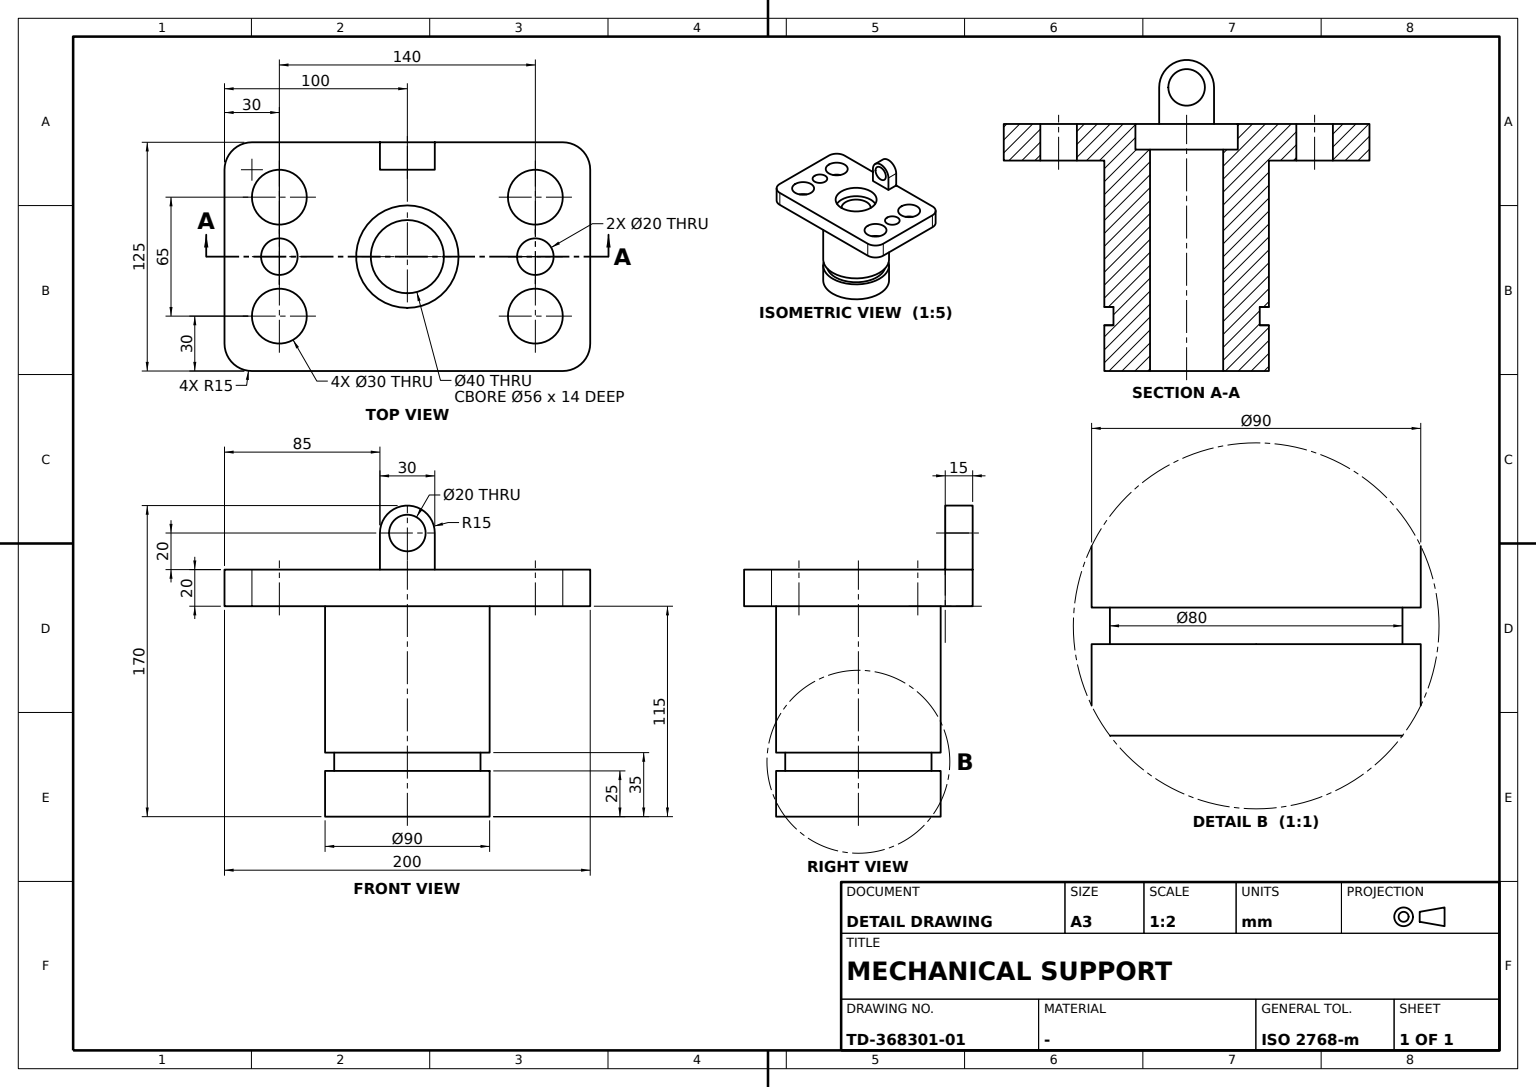
CATIA V5 part; units mm, degrees
sketch "Sketch1" plane through (0, 0, 0) normal (1, 0, 0) x (0, 1, 0)
  point P0 (20, 0)
  line L0 (20, 0) -> (20, 121)
  point P1 (45, 135)
  line L1 (45, 135) -> (45, 35)
  line L2 (45, 35) -> (40, 35)
  line L3 (40, 35) -> (40, 25)
  line L4 (40, 25) -> (45, 25)
  point P2 (45, 25)
  line L5 (45, 25) -> (45, 0)
  point P3 (45, 0)
  line L6 (45, 0) -> (20, 0)
  line L7 (20, 121) -> (28, 121)
  line L8 (28, 121) -> (28, 135)
  line L9 (28, 135) -> (45, 135)
  point P4 (45, 135)
  dimension "length L6" = 25
  dimension "distance L0 y axis" = 20
  dimension "length L5" = 25
  dimension "length L0" = 121
  dimension "length L3" = 10
  dimension "length L4" = 5
  dimension "distance L8 y axis" = 28
  dimension "distance L9 x axis" = 135
  constraint coincidence P0 x-axis
  constraint coincidence P2 L1
  constraint coincidence P3 x-axis
  constraint coincidence P4 L1
  constraint coincidence P1 P4
  constraint vertical L0 y-axis
  constraint vertical L1 y-axis
  constraint vertical L3 y-axis
  constraint vertical L5 y-axis
  constraint vertical L8 y-axis
  constraint horizontal L2 x-axis
  constraint horizontal L4 x-axis
  constraint horizontal L6 x-axis
  constraint horizontal L7 x-axis
  constraint horizontal L9 x-axis
revolve "Shaft1" add sketch "Sketch1" angle 360 about axis through (0, 0, 0) along (0, 0, 1)
sketch "Sketch2" plane through (0, 0, 135) normal (0, 0, 1) x (1, 0, 0)
  line L0 (100, 47.5) -> (100, -47.5)
  line L1 (85, -62.5) -> (-85, -62.5)
  line L2 (-100, -47.5) -> (-100, 47.5)
  line L3 (-85, 62.5) -> (85, 62.5)
  point P0 (100, 62.5)
  point P1 (100, -62.5)
  point P2 (-100, 62.5)
  circle A0 centre (70, -32.5) radius 15
  point P3 (70, -32.5)
  circle A1 centre (70, 0) radius 10
  point P4 (70, 0)
  circle A2 centre (70, 32.5) radius 15
  point P5 (70, 32.5)
  circle A3 centre (-70, 32.5) radius 15
  circle A4 centre (-70, 0) radius 10
  circle A5 centre (-70, -32.5) radius 15
  arc A6 (-85, 62.5) -> (-100, 47.5) centre (-85, 47.5) ccw
  arc A7 (85, 62.5) -> (100, 47.5) centre (85, 47.5) cw
  arc A8 (100, -47.5) -> (85, -62.5) centre (85, -47.5) cw
  arc A9 (-100, -47.5) -> (-85, -62.5) centre (-85, -47.5) ccw
  circle A10 centre (0, 0) radius 45
  dimension "radius A0" = 15
  dimension "distance P3 L1" = 30
  dimension "distance P3 L0" = 30
  dimension "radius A1" = 10
  dimension "distance P4 L0" = 30
  dimension "radius A2" = 15
  dimension "distance P5 L3" = 30
  dimension "distance P5 L0" = 30
  dimension "distance P2 P0" = 200
  dimension "radius A6" = 15
  dimension "distance P0 P1" = 125
  dimension "radius A7" = 15
  dimension "radius A8" = 15
  dimension "radius A9" = 15
  constraint vertical L0 y-axis
  constraint vertical L2 y-axis
  constraint horizontal L1 x-axis
  constraint horizontal L3 x-axis
  constraint equidistance L0 L2 origin
  constraint equidistance L1 L3 origin
  constraint coincidence P4 x-axis
  constraint coincidence L3 P2
  constraint coincidence L2 P2
  constraint coincidence L3 P0
  constraint coincidence L0 P0
  constraint coincidence L0 P1
  constraint coincidence L1 P1
  constraint symmetry A2 A3 y-axis
  constraint symmetry A1 A4 y-axis
  constraint symmetry A0 A5 y-axis
  constraint tangency A6 L3
  constraint tangency A6 L2
  constraint tangency A7 L3
  constraint tangency A7 L0
  constraint tangency A8 L0
  constraint tangency A8 L1
  constraint tangency A9 L2
  constraint tangency A9 L1
extrude "Pad1" add sketch "Sketch2" against normal blind 20
sketch "Sketch3" plane through (0, 62.5, 0) normal (0, 1, 0) x (-1, 0, 0)
  line L0 (15, 135) -> (15, 155)
  point P0 (15, 135)
  point P1 (15, 155)
  line L1 (-85, 135) -> (85, 135) construction
  point P2 (-15, 155)
  point P3 (-15, 135)
  line L2 (-15, 135) -> (-15, 155)
  line L3 (-15, 135) -> (15, 135)
  arc A0 (-15, 155) -> (15, 155) centre (0, 155) cw
  point P4 (15, 155)
  circle A1 centre (0, 155) radius 10
  dimension "length L0" = 20
  dimension "distance L0 y axis" = 15
  dimension "radius A1" = 10
  constraint vertical L0 y-axis
  constraint coincidence P0 L1
  constraint coincidence P4 L0
  constraint coincidence P4 P1
  constraint symmetry P1 P2 y-axis
  constraint symmetry P0 P3 y-axis
  constraint symmetry L0 L2 y-axis
  constraint horizontal L3 x-axis
  constraint tangency A0 L2
extrude "Pad2" add sketch "Sketch3" against normal blind 15
